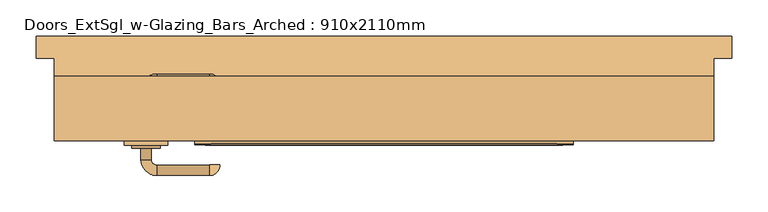
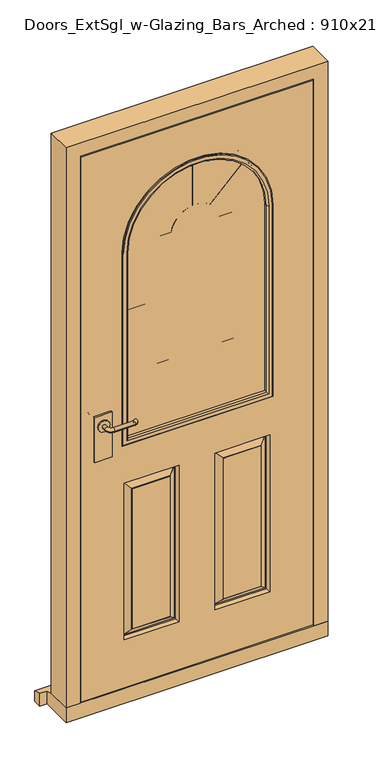
"""IFC4 building model written with IfcOpenShell, lengths in millimetres: door geometry, Doors_ExtSgl_w-Glazing_Bars_Arched : 910x2110mm."""

from ifc_helpers import new_model, si_unit, point, frame, frame_2d, origin, place, context, project, spatial, polyline, circle_curve, ellipse_curve, trimmed, segment, composite_curve, outline, extrude, faceted_brep, source, transform, mapped, element, save
from ifc_brep_helpers import plane_surface, cylinder_surface, revolved_surface, advanced_brep


def doors_extsgl_w_glazing_bars_arched_910x2110mm_1ab485ba(model_context):
    return source(origin(), model_context, "Body", "SolidModel", [
        extrude(outline(composite_curve([segment(trimmed(circle_curve(frame_2d((1050.0, -328.5)), 20.0), [point((1050.0, -348.5))], [point((1050.0, -308.5))], False, "CARTESIAN"), True, "CONTINUOUS"), segment(trimmed(circle_curve(frame_2d((1050.0, -328.5)), 20.0), [point((1050.0, -308.5))], [point((1050.0, -348.5))], False, "CARTESIAN"), True, "CONTINUOUS")], self_intersect=False)), frame((0.0, -22.9929895, 0.0), z_axis=(0.0, 1.0, 0.0), x_axis=(0.0, 0.0, 1.0)), (0.0, 0.0, 1.0), 4.5929895),
        advanced_brep(
        [(-321.5, -22.9929895, 1050.0), (-335.5, -22.9929895, 1050.0), (-335.5, -38.4, 1050.0), (-321.5, -38.4, 1050.0), (-313.5, -60.4, 1050.0), (-313.5, -46.4, 1050.0), (-241.5, -60.4, 1050.0), (-241.5, -46.4, 1050.0), (-240.5, -45.4, 1050.0), (-226.5, -45.4, 1050.0)],
        [
            (0, 1, circle_curve(frame((-328.5, -22.9929895, 1050.0), z_axis=(0.0, 1.0, 0.0), x_axis=(-1.0, 0.0, 0.0)), 7.0)),
            (1, 0, circle_curve(frame((-328.5, -22.9929895, 1050.0), z_axis=(0.0, 1.0, 0.0), x_axis=(-1.0, 0.0, 0.0)), 7.0)),
            (1, 2),
            (2, 3, circle_curve(frame((-328.5, -38.4, 1050.0), z_axis=(0.0, 1.0, 0.0), x_axis=(-1.0, 0.0, 0.0)), 7.0)),
            (3, 0),
            (3, 2, circle_curve(frame((-328.5, -38.4, 1050.0), z_axis=(0.0, 1.0, 0.0), x_axis=(-1.0, 0.0, 0.0)), 7.0)),
            (4, 5, circle_curve(frame((-313.5, -53.4, 1050.0), z_axis=(-1.0, 0.0, 0.0), x_axis=(0.0, -1.0, 0.0)), 7.0)),
            (5, 3, circle_curve(frame((-313.5, -38.4, 1050.0), z_axis=(0.0, 0.0, -1.0), x_axis=(-1.0, 0.0, 0.0)), 8.0)),
            (2, 4, circle_curve(frame((-313.5, -38.4, 1050.0), z_axis=(0.0, 0.0, 1.0), x_axis=(-1.0, 0.0, 0.0)), 22.0)),
            (5, 4, circle_curve(frame((-313.5, -53.4, 1050.0), z_axis=(-1.0, 0.0, 0.0), x_axis=(0.0, -1.0, 0.0)), 7.0)),
            (4, 6),
            (6, 7, circle_curve(frame((-241.5, -53.4, 1050.0), z_axis=(-1.0, 0.0, 0.0), x_axis=(0.0, -1.0, 0.0)), 7.0)),
            (7, 5),
            (7, 6, circle_curve(frame((-241.5, -53.4, 1050.0), z_axis=(-1.0, 0.0, 0.0), x_axis=(0.0, -1.0, 0.0)), 7.0)),
            (8, 9, circle_curve(frame((-233.5, -45.4, 1050.0), z_axis=(0.0, 1.0, 0.0), x_axis=(1.0, 0.0, 0.0)), 7.0)),
            (9, 8, circle_curve(frame((-233.5, -45.4, 1050.0), z_axis=(0.0, 1.0, 0.0), x_axis=(1.0, 0.0, 0.0)), 7.0)),
            (8, 7, circle_curve(frame((-241.5, -45.4, 1050.0), z_axis=(0.0, 0.0, -1.0), x_axis=(0.0, -1.0, 0.0)), 1.0)),
            (6, 9, circle_curve(frame((-241.5, -45.4, 1050.0), z_axis=(0.0, 0.0, 1.0), x_axis=(0.0, -1.0, 0.0)), 15.0)),
        ],
        [
            plane_surface(frame((-328.5, -22.9929895, 1050.0), z_axis=(0.0, 1.0, 0.0), x_axis=(0.0, 0.0, 1.0))),
            cylinder_surface(frame((-328.5, -22.9929895, 1050.0), z_axis=(0.0, 1.0, 0.0), x_axis=(-1.0, 0.0, 0.0)), 7.0),
            revolved_surface(trimmed(ellipse_curve(frame((-328.5, -38.4, 1050.0), z_axis=(0.0, -1.0, 0.0), x_axis=(-1.0, 0.0, 0.0)), 7.0, 7.0), [point((-321.5, -38.4, 1050.0))], [point((-335.5, -38.4, 1050.0))], True, "CARTESIAN"), (-313.5, -38.4, 1050.0), (0.0, 0.0, -1.0)),
            revolved_surface(trimmed(ellipse_curve(frame((-328.5, -38.4, 1050.0), z_axis=(0.0, -1.0, 0.0), x_axis=(-1.0, 0.0, 0.0)), 7.0, 7.0), [point((-335.5, -38.4, 1050.0))], [point((-321.5, -38.4, 1050.0))], True, "CARTESIAN"), (-313.5, -38.4, 1050.0), (0.0, 0.0, -1.0)),
            cylinder_surface(frame((-313.5, -53.4, 1050.0), z_axis=(-1.0, 0.0, 0.0), x_axis=(0.0, -1.0, 0.0)), 7.0),
            plane_surface(frame((-233.5, -45.4, 1050.0), z_axis=(0.0, 1.0, 0.0), x_axis=(0.0, 0.0, 1.0))),
            revolved_surface(trimmed(ellipse_curve(frame((-241.5, -53.4, 1050.0), z_axis=(1.0, 0.0, 0.0), x_axis=(0.0, -1.0, 0.0)), 7.0, 7.0), [point((-241.5, -46.4, 1050.0))], [point((-241.5, -60.4, 1050.0))], True, "CARTESIAN"), (-241.5, -45.4, 1050.0), (0.0, 0.0, -1.0)),
            revolved_surface(trimmed(ellipse_curve(frame((-241.5, -53.4, 1050.0), z_axis=(1.0, 0.0, 0.0), x_axis=(0.0, -1.0, 0.0)), 7.0, 7.0), [point((-241.5, -60.4, 1050.0))], [point((-241.5, -46.4, 1050.0))], True, "CARTESIAN"), (-241.5, -45.4, 1050.0), (0.0, 0.0, -1.0)),
        ],
        [
            (0, [[1, 2]]),
            (1, [[3, 4, 5, -2]]),
            (1, [[-5, 6, -3, -1]]),
            (2, [[7, 8, -4, 9]]),
            (3, [[10, -9, -6, -8]]),
            (4, [[11, 12, 13, -7]]),
            (4, [[-13, 14, -11, -10]]),
            (5, [[15, 16]]),
            (6, [[-15, 17, -12, 18]]),
            (7, [[-16, -18, -14, -17]]),
        ],
    ),
        extrude(outline(polyline([(-298.5, -12.4), (-298.5, -18.4), (-358.5, -18.4), (-358.5, -12.4), (-298.5, -12.4)])), frame((0.0, 0.0, 925.0), z_axis=(0.0, 0.0, 1.0), x_axis=(1.0, 0.0, 0.0)), (0.0, 0.0, 1.0), 165.0),
        extrude(outline(composite_curve([segment(trimmed(circle_curve(frame_2d((1050.0, -328.5)), 20.0), [point((1050.0, -348.5))], [point((1050.0, -308.5))], False, "CARTESIAN"), True, "CONTINUOUS"), segment(trimmed(circle_curve(frame_2d((1050.0, -328.5)), 20.0), [point((1050.0, -308.5))], [point((1050.0, -348.5))], False, "CARTESIAN"), True, "CONTINUOUS")], self_intersect=False)), frame((0.0, 37.6, 0.0), z_axis=(0.0, 1.0, 0.0), x_axis=(0.0, 0.0, 1.0)), (0.0, 0.0, 1.0), 4.5929895),
        advanced_brep(
        [(-321.5, 42.1929895, 1050.0), (-335.5, 42.1929895, 1050.0), (-321.5, 57.6, 1050.0), (-335.5, 57.6, 1050.0), (-313.5, 79.6, 1050.0), (-313.5, 65.6, 1050.0), (-241.5, 65.6, 1050.0), (-241.5, 79.6, 1050.0), (-240.5, 64.6, 1050.0), (-226.5, 64.6, 1050.0)],
        [
            (0, 1, circle_curve(frame((-328.5, 42.1929895, 1050.0), z_axis=(0.0, -1.0, 0.0), x_axis=(-1.0, 0.0, 0.0)), 7.0)),
            (1, 0, circle_curve(frame((-328.5, 42.1929895, 1050.0), z_axis=(0.0, -1.0, 0.0), x_axis=(-1.0, 0.0, 0.0)), 7.0)),
            (0, 2),
            (2, 3, circle_curve(frame((-328.5, 57.6, 1050.0), z_axis=(0.0, -1.0, 0.0), x_axis=(-1.0, 0.0, 0.0)), 7.0)),
            (3, 1),
            (3, 2, circle_curve(frame((-328.5, 57.6, 1050.0), z_axis=(0.0, -1.0, 0.0), x_axis=(-1.0, 0.0, 0.0)), 7.0)),
            (4, 3, circle_curve(frame((-313.5, 57.6, 1050.0), z_axis=(0.0, 0.0, 1.0), x_axis=(-1.0, 0.0, 0.0)), 22.0)),
            (2, 5, circle_curve(frame((-313.5, 57.6, 1050.0), z_axis=(0.0, 0.0, -1.0), x_axis=(-1.0, 0.0, 0.0)), 8.0)),
            (5, 4, circle_curve(frame((-313.5, 72.6, 1050.0), z_axis=(-1.0, 0.0, 0.0), x_axis=(0.0, 1.0, 0.0)), 7.0)),
            (4, 5, circle_curve(frame((-313.5, 72.6, 1050.0), z_axis=(-1.0, 0.0, 0.0), x_axis=(0.0, 1.0, 0.0)), 7.0)),
            (5, 6),
            (6, 7, circle_curve(frame((-241.5, 72.6, 1050.0), z_axis=(-1.0, 0.0, 0.0), x_axis=(0.0, 1.0, 0.0)), 7.0)),
            (7, 4),
            (7, 6, circle_curve(frame((-241.5, 72.6, 1050.0), z_axis=(-1.0, 0.0, 0.0), x_axis=(0.0, 1.0, 0.0)), 7.0)),
            (8, 9, circle_curve(frame((-233.5, 64.6, 1050.0), z_axis=(0.0, -1.0, 0.0), x_axis=(1.0, 0.0, 0.0)), 7.0)),
            (9, 8, circle_curve(frame((-233.5, 64.6, 1050.0), z_axis=(0.0, -1.0, 0.0), x_axis=(1.0, 0.0, 0.0)), 7.0)),
            (9, 7, circle_curve(frame((-241.5, 64.6, 1050.0), z_axis=(0.0, 0.0, 1.0), x_axis=(0.0, 1.0, 0.0)), 15.0)),
            (6, 8, circle_curve(frame((-241.5, 64.6, 1050.0), z_axis=(0.0, 0.0, -1.0), x_axis=(0.0, 1.0, 0.0)), 1.0)),
        ],
        [
            plane_surface(frame((-328.5, 42.1929895, 1050.0), z_axis=(0.0, -1.0, 0.0), x_axis=(0.0, 0.0, 1.0))),
            cylinder_surface(frame((-328.5, 42.1929895, 1050.0), z_axis=(0.0, -1.0, 0.0), x_axis=(-1.0, 0.0, 0.0)), 7.0),
            revolved_surface(trimmed(ellipse_curve(frame((-328.5, 57.6, 1050.0), z_axis=(0.0, -1.0, 0.0), x_axis=(-1.0, 0.0, 0.0)), 7.0, 7.0), [point((-321.5, 57.6, 1050.0))], [point((-335.5, 57.6, 1050.0))], True, "CARTESIAN"), (-313.5, 57.6, 1050.0), (0.0, 0.0, -1.0)),
            revolved_surface(trimmed(ellipse_curve(frame((-328.5, 57.6, 1050.0), z_axis=(0.0, -1.0, 0.0), x_axis=(-1.0, 0.0, 0.0)), 7.0, 7.0), [point((-335.5, 57.6, 1050.0))], [point((-321.5, 57.6, 1050.0))], True, "CARTESIAN"), (-313.5, 57.6, 1050.0), (0.0, 0.0, -1.0)),
            cylinder_surface(frame((-313.5, 72.6, 1050.0), z_axis=(-1.0, 0.0, 0.0), x_axis=(0.0, 1.0, 0.0)), 7.0),
            plane_surface(frame((-233.5, 64.6, 1050.0), z_axis=(0.0, -1.0, 0.0), x_axis=(0.0, 0.0, 1.0))),
            revolved_surface(trimmed(ellipse_curve(frame((-241.5, 72.6, 1050.0), z_axis=(-1.0, 0.0, 0.0), x_axis=(0.0, 1.0, 0.0)), 7.0, 7.0), [point((-241.5, 65.6, 1050.0))], [point((-241.5, 79.6, 1050.0))], True, "CARTESIAN"), (-241.5, 64.6, 1050.0), (0.0, 0.0, -1.0)),
            revolved_surface(trimmed(ellipse_curve(frame((-241.5, 72.6, 1050.0), z_axis=(-1.0, 0.0, 0.0), x_axis=(0.0, 1.0, 0.0)), 7.0, 7.0), [point((-241.5, 79.6, 1050.0))], [point((-241.5, 65.6, 1050.0))], True, "CARTESIAN"), (-241.5, 64.6, 1050.0), (0.0, 0.0, -1.0)),
        ],
        [
            (0, [[1, 2]]),
            (1, [[-1, 3, 4, 5]]),
            (1, [[-2, -5, 6, -3]]),
            (2, [[7, -4, 8, 9]]),
            (3, [[-8, -6, -7, 10]]),
            (4, [[-9, 11, 12, 13]]),
            (4, [[-10, -13, 14, -11]]),
            (5, [[15, 16]]),
            (6, [[17, -12, 18, -16]]),
            (7, [[-18, -14, -17, -15]]),
        ],
    ),
        extrude(outline(polyline([(-298.5, 31.6), (-358.5, 31.6), (-358.5, 37.6), (-298.5, 37.6), (-298.5, 31.6)])), frame((0.0, 0.0, 925.0), z_axis=(0.0, 0.0, 1.0), x_axis=(1.0, 0.0, 0.0)), (0.0, 0.0, 1.0), 165.0),
        faceted_brep([(384.5, 76.6, 54.5), (455.0, 76.6, 54.5), (455.0, -12.4, 54.5), (406.5, -12.4, 54.5), (406.5, 34.6, 54.5), (384.5, 34.6, 54.5), (384.5, 76.6, 2039.5), (-384.5, 76.6, 2039.5), (-384.5, 76.6, 54.5), (-455.0, 76.6, 54.5), (-455.0, 76.6, 2110.0), (455.0, 76.6, 2110.0), (455.0, -12.4, 2110.0), (-455.0, -12.4, 2110.0), (-455.0, -12.4, 54.5), (-406.5, -12.4, 54.5), (-406.5, -12.4, 2061.5), (406.5, -12.4, 2061.5), (406.5, 34.6, 2061.5), (-406.5, 34.6, 2061.5), (-406.5, 34.6, 54.5), (-384.5, 34.6, 54.5), (-384.5, 34.6, 2039.5), (384.5, 34.6, 2039.5)], [[[0, 1, 2, 3, 4, 5]], [[1, 0, 6, 7, 8, 9, 10, 11]], [[2, 1, 11, 12]], [[3, 2, 12, 13, 14, 15, 16, 17]], [[4, 3, 17, 18]], [[5, 4, 18, 19, 20, 21, 22, 23]], [[0, 5, 23, 6]], [[8, 7, 22, 21]], [[9, 8, 21, 20, 15, 14]], [[10, 9, 14, 13]], [[16, 15, 20, 19]], [[11, 10, 13, 12]], [[17, 16, 19, 18]], [[7, 6, 23, 22]]]),
        advanced_brep(
        [(403.5, -12.4, 58.5), (403.5, -12.4, 2058.5), (-404.4250294, -12.4, 2058.5), (-404.4250294, -12.4, 58.5), (-253.5, -12.4, 958.5), (-253.5, -12.4, 1655.0), (253.5, -12.4, 1655.0), (253.5, -12.4, 958.5), (-62.5, -12.4, 808.5), (-62.5, -12.4, 233.5), (-253.5, -12.4, 233.5), (-253.5, -12.4, 808.5), (253.5, -12.4, 808.5), (253.5, -12.4, 233.5), (62.5, -12.4, 233.5), (62.5, -12.4, 808.5), (-92.5, -12.4, 263.5), (-92.5, -12.4, 778.5), (-223.5, -12.4, 778.5), (-223.5, -12.4, 263.5), (223.5, -12.4, 263.5), (223.5, -12.4, 778.5), (92.5, -12.4, 778.5), (92.5, -12.4, 263.5), (403.5, 31.6, 58.5), (-404.4250294, 31.6, 58.5), (-404.4250294, 31.6, 2058.5), (403.5, 31.6, 2058.5), (-253.5, 31.6, 958.5), (253.5, 31.6, 958.5), (253.5, 31.6, 1655.0), (-253.5, 31.6, 1655.0), (62.5, 31.6, 808.5), (62.5, 31.6, 233.5), (253.5, 31.6, 233.5), (253.5, 31.6, 808.5), (-253.5, 31.6, 808.5), (-253.5, 31.6, 233.5), (-62.5, 31.6, 233.5), (-62.5, 31.6, 808.5), (92.5, 31.6, 263.5), (92.5, 31.6, 778.5), (223.5, 31.6, 778.5), (223.5, 31.6, 263.5), (-223.5, 31.6, 263.5), (-223.5, 31.6, 778.5), (-92.5, 31.6, 778.5), (-92.5, 31.6, 263.5), (65.5, 16.6, 805.5), (65.5, 16.6, 236.5), (90.5, 30.6, 780.5), (90.5, 30.6, 261.5), (70.5, 16.6, 241.5), (70.5, 16.6, 800.5), (92.5, 30.6, 263.5), (92.5, 30.6, 778.5), (250.5, 16.6, 236.5), (225.5, 30.6, 261.5), (245.5, 16.6, 241.5), (223.5, 30.6, 263.5), (250.5, 16.6, 805.5), (225.5, 30.6, 780.5), (245.5, 16.6, 800.5), (223.5, 30.6, 778.5), (-250.5, 16.6, 805.5), (-250.5, 16.6, 236.5), (-225.5, 30.6, 780.5), (-225.5, 30.6, 261.5), (-245.5, 16.6, 241.5), (-245.5, 16.6, 800.5), (-223.5, 30.6, 263.5), (-223.5, 30.6, 778.5), (-65.5, 16.6, 236.5), (-90.5, 30.6, 261.5), (-70.5, 16.6, 241.5), (-92.5, 30.6, 263.5), (-65.5, 16.6, 805.5), (-90.5, 30.6, 780.5), (-70.5, 16.6, 800.5), (-92.5, 30.6, 778.5), (-92.5, -11.4, 263.5), (-92.5, -11.4, 778.5), (-70.5, 2.6, 241.5), (-70.5, 2.6, 800.5), (-90.5, -11.4, 780.5), (-90.5, -11.4, 261.5), (-65.5, 2.6, 805.5), (-65.5, 2.6, 236.5), (-223.5, -11.4, 778.5), (-245.5, 2.6, 800.5), (-225.5, -11.4, 780.5), (-250.5, 2.6, 805.5), (-223.5, -11.4, 263.5), (-245.5, 2.6, 241.5), (-225.5, -11.4, 261.5), (-250.5, 2.6, 236.5), (250.5, 2.6, 805.5), (250.5, 2.6, 236.5), (225.5, -11.4, 780.5), (225.5, -11.4, 261.5), (245.5, 2.6, 241.5), (245.5, 2.6, 800.5), (223.5, -11.4, 263.5), (223.5, -11.4, 778.5), (65.5, 2.6, 236.5), (90.5, -11.4, 261.5), (70.5, 2.6, 241.5), (92.5, -11.4, 263.5), (65.5, 2.6, 805.5), (90.5, -11.4, 780.5), (70.5, 2.6, 800.5), (92.5, -11.4, 778.5)],
        [
            (0, 1),
            (1, 2),
            (2, 3),
            (3, 0),
            (4, 5),
            (5, 6, circle_curve(frame((0.0, -12.4, 1655.0), z_axis=(0.0, 1.0, 0.0), x_axis=(1.0, 0.0, 0.0)), 253.5)),
            (6, 7),
            (7, 4),
            (8, 9),
            (9, 10),
            (10, 11),
            (11, 8),
            (12, 13),
            (13, 14),
            (14, 15),
            (15, 12),
            (16, 17),
            (17, 18),
            (18, 19),
            (19, 16),
            (20, 21),
            (21, 22),
            (22, 23),
            (23, 20),
            (24, 25),
            (25, 26),
            (26, 27),
            (27, 24),
            (28, 29),
            (29, 30),
            (30, 31, circle_curve(frame((0.0, 31.6, 1655.0), z_axis=(0.0, -1.0, 0.0), x_axis=(1.0, 0.0, 0.0)), 253.5)),
            (31, 28),
            (32, 33),
            (33, 34),
            (34, 35),
            (35, 32),
            (36, 37),
            (37, 38),
            (38, 39),
            (39, 36),
            (40, 41),
            (41, 42),
            (42, 43),
            (43, 40),
            (44, 45),
            (45, 46),
            (46, 47),
            (47, 44),
            (0, 24),
            (27, 1),
            (26, 2),
            (25, 3),
            (4, 28),
            (31, 5),
            (30, 6),
            (29, 7),
            (48, 49),
            (49, 33),
            (32, 48),
            (50, 51),
            (51, 52),
            (52, 53),
            (53, 50),
            (40, 54),
            (54, 55),
            (55, 41),
            (49, 56),
            (56, 34),
            (51, 57),
            (57, 58),
            (58, 52),
            (43, 59),
            (59, 54),
            (56, 60),
            (60, 35),
            (57, 61),
            (61, 62),
            (62, 58),
            (42, 63),
            (63, 59),
            (60, 48),
            (62, 53),
            (61, 50),
            (63, 55),
            (64, 65),
            (65, 37),
            (36, 64),
            (66, 67),
            (67, 68),
            (68, 69),
            (69, 66),
            (44, 70),
            (70, 71),
            (71, 45),
            (65, 72),
            (72, 38),
            (67, 73),
            (73, 74),
            (74, 68),
            (47, 75),
            (75, 70),
            (72, 76),
            (76, 39),
            (73, 77),
            (77, 78),
            (78, 74),
            (46, 79),
            (79, 75),
            (76, 64),
            (78, 69),
            (77, 66),
            (79, 71),
            (80, 81),
            (81, 17),
            (16, 80),
            (82, 83),
            (83, 84),
            (84, 85),
            (85, 82),
            (8, 86),
            (86, 87),
            (87, 9),
            (81, 88),
            (88, 18),
            (83, 89),
            (89, 90),
            (90, 84),
            (11, 91),
            (91, 86),
            (88, 92),
            (92, 19),
            (89, 93),
            (93, 94),
            (94, 90),
            (10, 95),
            (95, 91),
            (92, 80),
            (94, 85),
            (93, 82),
            (95, 87),
            (96, 97),
            (97, 13),
            (12, 96),
            (98, 99),
            (99, 100),
            (100, 101),
            (101, 98),
            (20, 102),
            (102, 103),
            (103, 21),
            (97, 104),
            (104, 14),
            (99, 105),
            (105, 106),
            (106, 100),
            (23, 107),
            (107, 102),
            (104, 108),
            (108, 15),
            (105, 109),
            (109, 110),
            (110, 106),
            (22, 111),
            (111, 107),
            (108, 96),
            (110, 101),
            (109, 98),
            (111, 103),
        ],
        [
            plane_surface(frame((403.5, -12.4, 58.5), z_axis=(0.0, -1.0, 0.0), x_axis=(0.0, 0.0, 1.0))),
            plane_surface(frame((403.5, 31.6, 58.5), z_axis=(0.0, 1.0, 0.0), x_axis=(0.0, 0.0, -1.0))),
            plane_surface(frame((403.5, -12.4, 58.5), z_axis=(1.0, 0.0, 0.0), x_axis=(0.0, 1.0, 0.0))),
            plane_surface(frame((403.5, -12.4, 2058.5), z_axis=(0.0, 0.0, 1.0), x_axis=(0.0, 1.0, 0.0))),
            plane_surface(frame((-404.4250294, -12.4, 2058.5), z_axis=(-1.0, 0.0, 0.0), x_axis=(0.0, 1.0, 0.0))),
            plane_surface(frame((-404.4250294, -12.4, 58.5), z_axis=(0.0, 0.0, -1.0), x_axis=(0.0, 1.0, 0.0))),
            plane_surface(frame((-253.5, -12.4, 958.5), z_axis=(1.0, 0.0, 0.0), x_axis=(0.0, 1.0, 0.0))),
            revolved_surface(polyline([(253.5, 31.6, 1655.0), (253.5, -12.4, 1655.0)]), (0.0, -12.4, 1655.0), (0.0, 1.0, 0.0)),
            plane_surface(frame((253.5, -12.4, 1655.0), z_axis=(-1.0, 0.0, 0.0), x_axis=(0.0, 1.0, 0.0))),
            plane_surface(frame((253.5, -12.4, 958.5), z_axis=(0.0, 0.0, 1.0), x_axis=(0.0, 1.0, 0.0))),
            plane_surface(frame((62.5, 31.6, 808.5), z_axis=(0.9805806756909202, 0.19611613513818407, 0.0), x_axis=(0.0, 0.0, -1.0))),
            plane_surface(frame((70.5, 16.6, 800.5), z_axis=(-0.5734623443633278, 0.8192319205190408, 0.0), x_axis=(0.0, 0.0, -1.0))),
            plane_surface(frame((92.5, 30.6, 778.5), z_axis=(-1.0, 0.0, 0.0), x_axis=(0.0, 0.0, -1.0))),
            plane_surface(frame((62.5, 31.6, 233.5), z_axis=(0.0, 0.19611613513818724, 0.9805806756909196), x_axis=(1.0, 0.0, 0.0))),
            plane_surface(frame((70.5, 16.6, 241.5), z_axis=(0.0, 0.819231920519039, -0.5734623443633305), x_axis=(1.0, 0.0, 0.0))),
            plane_surface(frame((92.5, 30.6, 263.5), z_axis=(0.0, 0.0, -1.0), x_axis=(1.0, 0.0, 0.0))),
            plane_surface(frame((253.5, 31.6, 233.5), z_axis=(-0.9805806756909189, 0.19611613513819037, 0.0), x_axis=(0.0, 0.0, 1.0))),
            plane_surface(frame((245.5, 16.6, 241.5), z_axis=(0.5734623443633332, 0.819231920519037, 0.0), x_axis=(0.0, 0.0, 1.0))),
            plane_surface(frame((223.5, 30.6, 263.5), z_axis=(1.0, 0.0, 0.0), x_axis=(0.0, 0.0, 1.0))),
            plane_surface(frame((253.5, 31.6, 808.5), z_axis=(0.0, 0.1961161351381872, -0.9805806756909196), x_axis=(-1.0, 0.0, 0.0))),
            plane_surface(frame((250.5, 16.6, 805.5), z_axis=(0.0, 1.0, 0.0), x_axis=(-1.0, 0.0, 0.0))),
            plane_surface(frame((245.5, 16.6, 800.5), z_axis=(0.0, 0.8192319205190389, 0.5734623443633305), x_axis=(-1.0, 0.0, 0.0))),
            plane_surface(frame((225.5, 30.6, 780.5), z_axis=(0.0, 1.0, 0.0), x_axis=(-1.0, 0.0, 0.0))),
            plane_surface(frame((223.5, 30.6, 778.5), z_axis=(0.0, 0.0, 1.0), x_axis=(-1.0, 0.0, 0.0))),
            plane_surface(frame((-253.5, 31.6, 808.5), z_axis=(0.9805806756909202, 0.19611613513818407, 0.0), x_axis=(0.0, 0.0, -1.0))),
            plane_surface(frame((-245.5, 16.6, 800.5), z_axis=(-0.5734623443633278, 0.8192319205190408, 0.0), x_axis=(0.0, 0.0, -1.0))),
            plane_surface(frame((-223.5, 30.6, 778.5), z_axis=(-1.0, 0.0, 0.0), x_axis=(0.0, 0.0, -1.0))),
            plane_surface(frame((-253.5, 31.6, 233.5), z_axis=(0.0, 0.19611613513818724, 0.9805806756909196), x_axis=(1.0, 0.0, 0.0))),
            plane_surface(frame((-245.5, 16.6, 241.5), z_axis=(0.0, 0.819231920519039, -0.5734623443633305), x_axis=(1.0, 0.0, 0.0))),
            plane_surface(frame((-223.5, 30.6, 263.5), z_axis=(0.0, 0.0, -1.0), x_axis=(1.0, 0.0, 0.0))),
            plane_surface(frame((-62.5, 31.6, 233.5), z_axis=(-0.9805806756909189, 0.1961161351381904, 0.0), x_axis=(0.0, 0.0, 1.0))),
            plane_surface(frame((-70.5, 16.6, 241.5), z_axis=(0.5734623443633332, 0.8192319205190371, 0.0), x_axis=(0.0, 0.0, 1.0))),
            plane_surface(frame((-92.5, 30.6, 263.5), z_axis=(1.0, 0.0, 0.0), x_axis=(0.0, 0.0, 1.0))),
            plane_surface(frame((-62.5, 31.6, 808.5), z_axis=(0.0, 0.19611613513818724, -0.9805806756909196), x_axis=(-1.0, 0.0, 0.0))),
            plane_surface(frame((-65.5, 16.6, 805.5), z_axis=(0.0, 1.0, 0.0), x_axis=(-1.0, 0.0, 0.0))),
            plane_surface(frame((-70.5, 16.6, 800.5), z_axis=(0.0, 0.819231920519039, 0.5734623443633305), x_axis=(-1.0, 0.0, 0.0))),
            plane_surface(frame((-90.5, 30.6, 780.5), z_axis=(0.0, 1.0, 0.0), x_axis=(-1.0, 0.0, 0.0))),
            plane_surface(frame((-92.5, 30.6, 778.5), z_axis=(0.0, 0.0, 1.0), x_axis=(-1.0, 0.0, 0.0))),
            plane_surface(frame((-92.5, -12.4, 263.5), z_axis=(1.0, 0.0, 0.0), x_axis=(0.0, 0.0, 1.0))),
            plane_surface(frame((-90.5, -11.4, 261.5), z_axis=(0.5734623443633226, -0.8192319205190446, 0.0), x_axis=(0.0, 0.0, 1.0))),
            plane_surface(frame((-65.5, 2.6, 236.5), z_axis=(-0.9805806756909214, -0.19611613513817774, 0.0), x_axis=(0.0, 0.0, 1.0))),
            plane_surface(frame((-92.5, -12.4, 778.5), z_axis=(0.0, 0.0, 1.0), x_axis=(-1.0, 0.0, 0.0))),
            plane_surface(frame((-90.5, -11.4, 780.5), z_axis=(0.0, -0.8192319205190427, 0.5734623443633252), x_axis=(-1.0, 0.0, 0.0))),
            plane_surface(frame((-65.5, 2.6, 805.5), z_axis=(0.0, -0.1961161351381809, -0.9805806756909208), x_axis=(-1.0, 0.0, 0.0))),
            plane_surface(frame((-223.5, -12.4, 778.5), z_axis=(-1.0, 0.0, 0.0), x_axis=(0.0, 0.0, -1.0))),
            plane_surface(frame((-225.5, -11.4, 780.5), z_axis=(-0.5734623443633279, -0.8192319205190408, 0.0), x_axis=(0.0, 0.0, -1.0))),
            plane_surface(frame((-250.5, 2.6, 805.5), z_axis=(0.9805806756909202, -0.1961161351381841, 0.0), x_axis=(0.0, 0.0, -1.0))),
            plane_surface(frame((-223.5, -12.4, 263.5), z_axis=(0.0, 0.0, -1.0), x_axis=(1.0, 0.0, 0.0))),
            plane_surface(frame((-223.5, -11.4, 263.5), z_axis=(0.0, -1.0, 0.0), x_axis=(1.0, 0.0, 0.0))),
            plane_surface(frame((-225.5, -11.4, 261.5), z_axis=(0.0, -0.8192319205190427, -0.5734623443633252), x_axis=(1.0, 0.0, 0.0))),
            plane_surface(frame((-245.5, 2.6, 241.5), z_axis=(0.0, -1.0, 0.0), x_axis=(1.0, 0.0, 0.0))),
            plane_surface(frame((-250.5, 2.6, 236.5), z_axis=(0.0, -0.19611613513818094, 0.9805806756909209), x_axis=(1.0, 0.0, 0.0))),
            plane_surface(frame((253.5, -12.4, 808.5), z_axis=(-0.9805806756909202, -0.19611613513818407, 0.0), x_axis=(0.0, 0.0, -1.0))),
            plane_surface(frame((245.5, 2.6, 800.5), z_axis=(0.5734623443633278, -0.8192319205190408, 0.0), x_axis=(0.0, 0.0, -1.0))),
            plane_surface(frame((223.5, -11.4, 778.5), z_axis=(1.0, 0.0, 0.0), x_axis=(0.0, 0.0, -1.0))),
            plane_surface(frame((253.5, -12.4, 233.5), z_axis=(0.0, -0.19611613513818724, 0.9805806756909196), x_axis=(-1.0, 0.0, 0.0))),
            plane_surface(frame((245.5, 2.6, 241.5), z_axis=(0.0, -0.819231920519039, -0.5734623443633305), x_axis=(-1.0, 0.0, 0.0))),
            plane_surface(frame((223.5, -11.4, 263.5), z_axis=(0.0, 0.0, -1.0), x_axis=(-1.0, 0.0, 0.0))),
            plane_surface(frame((62.5, -12.4, 233.5), z_axis=(0.9805806756909189, -0.19611613513819046, 0.0), x_axis=(0.0, 0.0, 1.0))),
            plane_surface(frame((70.5, 2.6, 241.5), z_axis=(-0.5734623443633331, -0.8192319205190371, 0.0), x_axis=(0.0, 0.0, 1.0))),
            plane_surface(frame((92.5, -11.4, 263.5), z_axis=(-1.0, 0.0, 0.0), x_axis=(0.0, 0.0, 1.0))),
            plane_surface(frame((62.5, -12.4, 808.5), z_axis=(0.0, -0.1961161351381873, -0.9805806756909196), x_axis=(1.0, 0.0, 0.0))),
            plane_surface(frame((65.5, 2.6, 805.5), z_axis=(0.0, -1.0, 0.0), x_axis=(1.0, 0.0, 0.0))),
            plane_surface(frame((70.5, 2.6, 800.5), z_axis=(0.0, -0.819231920519039, 0.5734623443633304), x_axis=(1.0, 0.0, 0.0))),
            plane_surface(frame((90.5, -11.4, 780.5), z_axis=(0.0, -1.0, 0.0), x_axis=(1.0, 0.0, 0.0))),
            plane_surface(frame((92.5, -11.4, 778.5), z_axis=(0.0, 0.0, 1.0), x_axis=(1.0, 0.0, 0.0))),
        ],
        [
            (0, [[1, 2, 3, 4], [5, 6, 7, 8], [9, 10, 11, 12], [13, 14, 15, 16]]),
            (0, [[17, 18, 19, 20]]),
            (0, [[21, 22, 23, 24]]),
            (1, [[25, 26, 27, 28], [29, 30, 31, 32], [33, 34, 35, 36], [37, 38, 39, 40]]),
            (1, [[41, 42, 43, 44]]),
            (1, [[45, 46, 47, 48]]),
            (2, [[-1, 49, -28, 50]]),
            (3, [[-2, -50, -27, 51]]),
            (4, [[-3, -51, -26, 52]]),
            (5, [[-4, -52, -25, -49]]),
            (6, [[-5, 53, -32, 54]]),
            (7, [[-6, -54, -31, 55]]),
            (8, [[-7, -55, -30, 56]]),
            (9, [[-8, -56, -29, -53]]),
            (10, [[57, 58, -33, 59]]),
            (11, [[60, 61, 62, 63]]),
            (12, [[64, 65, 66, -41]]),
            (13, [[-58, 67, 68, -34]]),
            (14, [[-61, 69, 70, 71]]),
            (15, [[-64, -44, 72, 73]]),
            (16, [[-68, 74, 75, -35]]),
            (17, [[-70, 76, 77, 78]]),
            (18, [[-72, -43, 79, 80]]),
            (19, [[-59, -36, -75, 81]]),
            (20, [[-57, -81, -74, -67], [-62, -71, -78, 82]]),
            (21, [[-63, -82, -77, 83]]),
            (22, [[-60, -83, -76, -69], [-65, -73, -80, 84]]),
            (23, [[-66, -84, -79, -42]]),
            (24, [[85, 86, -37, 87]]),
            (25, [[88, 89, 90, 91]]),
            (26, [[92, 93, 94, -45]]),
            (27, [[-86, 95, 96, -38]]),
            (28, [[-89, 97, 98, 99]]),
            (29, [[-92, -48, 100, 101]]),
            (30, [[-96, 102, 103, -39]]),
            (31, [[-98, 104, 105, 106]]),
            (32, [[-100, -47, 107, 108]]),
            (33, [[-87, -40, -103, 109]]),
            (34, [[-85, -109, -102, -95], [-90, -99, -106, 110]]),
            (35, [[-91, -110, -105, 111]]),
            (36, [[-88, -111, -104, -97], [-93, -101, -108, 112]]),
            (37, [[-94, -112, -107, -46]]),
            (38, [[113, 114, -17, 115]]),
            (39, [[116, 117, 118, 119]]),
            (40, [[120, 121, 122, -9]]),
            (41, [[-114, 123, 124, -18]]),
            (42, [[-117, 125, 126, 127]]),
            (43, [[-120, -12, 128, 129]]),
            (44, [[-124, 130, 131, -19]]),
            (45, [[-126, 132, 133, 134]]),
            (46, [[-128, -11, 135, 136]]),
            (47, [[-115, -20, -131, 137]]),
            (48, [[-118, -127, -134, 138], [-113, -137, -130, -123]]),
            (49, [[-119, -138, -133, 139]]),
            (50, [[-121, -129, -136, 140], [-116, -139, -132, -125]]),
            (51, [[-122, -140, -135, -10]]),
            (52, [[141, 142, -13, 143]]),
            (53, [[144, 145, 146, 147]]),
            (54, [[148, 149, 150, -21]]),
            (55, [[-142, 151, 152, -14]]),
            (56, [[-145, 153, 154, 155]]),
            (57, [[-148, -24, 156, 157]]),
            (58, [[-152, 158, 159, -15]]),
            (59, [[-154, 160, 161, 162]]),
            (60, [[-156, -23, 163, 164]]),
            (61, [[-143, -16, -159, 165]]),
            (62, [[-141, -165, -158, -151], [-146, -155, -162, 166]]),
            (63, [[-147, -166, -161, 167]]),
            (64, [[-144, -167, -160, -153], [-149, -157, -164, 168]]),
            (65, [[-150, -168, -163, -22]]),
        ],
    ),
        faceted_brep([(480.0, 131.6, 0.0), (480.0, 131.6, 38.5947221), (480.0, 101.6, 47.2703282), (480.0, 101.6, 0.0), (-480.0, 131.6, 38.5947221), (-480.0, 131.6, 0.0), (-480.0, 101.6, 0.0), (-480.0, 101.6, 47.2703282), (455.0, 101.6, 0.0), (455.0, -12.4, 0.0), (-455.0, -12.4, 0.0), (-455.0, 101.6, 0.0), (-455.0, 101.6, 47.2703282), (-455.0, 76.6, 54.5), (455.0, 76.6, 54.5), (455.0, 101.6, 47.2703282), (-455.0, -12.4, 54.5), (455.0, -12.4, 54.5)], [[[0, 1, 2, 3]], [[4, 5, 6, 7]], [[5, 0, 3, 8, 9, 10, 11, 6]], [[1, 0, 5, 4]], [[1, 4, 7, 12, 13, 14, 15, 2]], [[13, 16, 17, 14]], [[16, 10, 9, 17]], [[12, 11, 10, 16, 13]], [[11, 12, 7, 6]], [[8, 15, 14, 17, 9]], [[15, 8, 3, 2]]]),
        extrude(outline(composite_curve([segment(polyline([(958.5, -253.5), (958.5, 253.5), (1655.0, 253.5)]), True, "CONTINUOUS"), segment(trimmed(circle_curve(frame_2d((1655.0, 0.0)), 253.5), [point((1655.0, 253.5))], [point((1655.0, -253.5))], False, "CARTESIAN"), True, "CONTINUOUS"), segment(polyline([(1655.0, -253.5), (958.5, -253.5)]), True, "CONTINUOUS")], self_intersect=False)), frame((0.0, -2.4, 0.0), z_axis=(0.0, 1.0, 0.0), x_axis=(0.0, 0.0, 1.0)), (0.0, 0.0, 1.0), 24.0),
        advanced_brep(
        [(-261.5, 35.6, 950.5), (-261.5, 31.6, 950.5), (-261.5, 31.6, 1655.0), (-261.5, 35.6, 1655.0), (-259.5, 37.6, 952.5), (-259.5, 37.6, 1655.0), (-241.5, 32.6, 970.5), (-246.5, 37.6, 965.5), (-246.5, 37.6, 1655.0), (-241.5, 32.6, 1655.0), (-241.5, 21.6, 970.5), (-241.5, 21.6, 1655.0), (-253.5, 31.6, 958.5), (-253.5, 21.6, 958.5), (-253.5, 21.6, 1655.0), (-253.5, 31.6, 1655.0), (261.5, 35.6, 1655.0), (261.5, 31.6, 1655.0), (259.5, 37.6, 1655.0), (259.5, 37.6, 952.5), (246.5, 37.6, 1655.0), (246.5, 37.6, 965.5), (241.5, 32.6, 1655.0), (241.5, 21.6, 1655.0), (253.5, 21.6, 1655.0), (253.5, 21.6, 958.5), (241.5, 21.6, 970.5), (253.5, 31.6, 1655.0), (261.5, 31.6, 950.5), (253.5, 31.6, 958.5), (261.5, 35.6, 950.5), (241.5, 32.6, 970.5)],
        [
            (0, 1),
            (1, 2),
            (2, 3),
            (3, 0),
            (4, 0, ellipse_curve(frame((-259.5, 35.6, 952.5), z_axis=(-0.7071067811865475, 0.0, 0.7071067811865475), x_axis=(-0.7071067811865472, 0.0, -0.7071067811865477)), 2.8284271, 2.0)),
            (3, 5, circle_curve(frame((-259.5, 35.6, 1655.0), z_axis=(0.0, 0.0, -1.0), x_axis=(-1.0, 0.0, 0.0)), 2.0)),
            (5, 4),
            (6, 7, ellipse_curve(frame((-246.5, 32.6, 965.5), z_axis=(-0.7071067811865475, 0.0, 0.7071067811865475), x_axis=(-0.7071067811865472, 0.0, -0.7071067811865477)), 7.0710678, 5.0)),
            (7, 8),
            (8, 9, circle_curve(frame((-246.5, 32.6, 1655.0), z_axis=(0.0, 0.0, -1.0), x_axis=(-1.0, 0.0, 0.0)), 5.0)),
            (9, 6),
            (10, 6),
            (9, 11),
            (11, 10),
            (12, 13),
            (13, 14),
            (14, 15),
            (15, 12),
            (16, 3, circle_curve(frame((0.0, 35.6, 1655.0), z_axis=(0.0, -1.0, 0.0), x_axis=(-1.0, 0.0, 0.0)), 261.5)),
            (2, 17, circle_curve(frame((0.0, 31.6, 1655.0), z_axis=(0.0, 1.0, 0.0), x_axis=(-1.0, 0.0, 0.0)), 261.5)),
            (17, 16),
            (18, 5, circle_curve(frame((0.0, 37.6, 1655.0), z_axis=(0.0, -1.0, 0.0), x_axis=(-1.0, 0.0, 0.0)), 259.5)),
            (16, 18, circle_curve(frame((259.5, 35.6, 1655.0), z_axis=(0.0, 0.0, 1.0), x_axis=(1.0, 0.0, 0.0)), 2.0)),
            (18, 19),
            (19, 4),
            (20, 8, circle_curve(frame((0.0, 37.6, 1655.0), z_axis=(0.0, -1.0, 0.0), x_axis=(-1.0, 0.0, 0.0)), 246.5)),
            (7, 21),
            (21, 20),
            (22, 9, circle_curve(frame((0.0, 32.6, 1655.0), z_axis=(0.0, -1.0, 0.0), x_axis=(-1.0, 0.0, 0.0)), 241.5)),
            (20, 22, circle_curve(frame((246.5, 32.6, 1655.0), z_axis=(0.0, 0.0, 1.0), x_axis=(1.0, 0.0, 0.0)), 5.0)),
            (23, 11, circle_curve(frame((0.0, 21.6, 1655.0), z_axis=(0.0, -1.0, 0.0), x_axis=(-1.0, 0.0, 0.0)), 241.5)),
            (22, 23),
            (24, 14, circle_curve(frame((0.0, 21.6, 1655.0), z_axis=(0.0, -1.0, 0.0), x_axis=(-1.0, 0.0, 0.0)), 253.5)),
            (13, 25),
            (25, 24),
            (23, 26),
            (26, 10),
            (27, 15, circle_curve(frame((0.0, 31.6, 1655.0), z_axis=(0.0, -1.0, 0.0), x_axis=(-1.0, 0.0, 0.0)), 253.5)),
            (24, 27),
            (1, 28),
            (28, 17),
            (27, 29),
            (29, 12),
            (28, 30),
            (30, 16),
            (30, 19, ellipse_curve(frame((259.5, 35.6, 952.5), z_axis=(0.7071067811865475, 0.0, 0.7071067811865475), x_axis=(-0.7071067811865475, 0.0, 0.7071067811865476)), 2.8284271, 2.0)),
            (21, 31, ellipse_curve(frame((246.5, 32.6, 965.5), z_axis=(0.7071067811865475, 0.0, 0.7071067811865475), x_axis=(-0.7071067811865475, 0.0, 0.7071067811865476)), 7.0710678, 5.0)),
            (31, 22),
            (31, 26),
            (25, 29),
            (0, 30),
            (6, 31),
        ],
        [
            plane_surface(frame((-261.5, 31.6, 950.5), z_axis=(-1.0, 0.0, 0.0), x_axis=(0.0, 0.0, 1.0))),
            cylinder_surface(frame((-259.5, 35.6, 958.5), z_axis=(0.0, 0.0, -1.0), x_axis=(-1.0, 0.0, 0.0)), 2.0),
            cylinder_surface(frame((-246.5, 32.6, 958.5), z_axis=(0.0, 0.0, -1.0), x_axis=(-1.0, 0.0, 0.0)), 5.0),
            plane_surface(frame((-241.5, 32.6, 970.5), z_axis=(1.0, 0.0, 0.0), x_axis=(0.0, 0.0, 1.0))),
            plane_surface(frame((-253.5, 21.6, 958.5), z_axis=(-1.0, 0.0, 0.0), x_axis=(0.0, 0.0, 1.0))),
            cylinder_surface(frame((0.0, 31.6, 1655.0), z_axis=(0.0, 1.0, 0.0), x_axis=(-1.0, 0.0, 0.0)), 261.5),
            revolved_surface(trimmed(ellipse_curve(frame((-259.5, 35.6, 1655.0), z_axis=(0.0, 0.0, -1.0), x_axis=(-1.0, 0.0, 0.0)), 2.0, 2.0), [point((-261.5, 35.6, 1655.0))], [point((-259.5, 37.6, 1655.0))], True, "CARTESIAN"), (0.0, 31.6, 1655.0), (0.0, 1.0, 0.0)),
            plane_surface(frame((0.0, 37.6, 1655.0), z_axis=(0.0, 1.0, 0.0), x_axis=(-1.0, 0.0, 0.0))),
            revolved_surface(trimmed(ellipse_curve(frame((-246.5, 32.6, 1655.0), z_axis=(0.0, 0.0, -1.0), x_axis=(-1.0, 0.0, 0.0)), 5.0, 5.0), [point((-246.5, 37.6, 1655.0))], [point((-241.5, 32.6, 1655.0))], True, "CARTESIAN"), (0.0, 31.6, 1655.0), (0.0, 1.0, 0.0)),
            revolved_surface(polyline([(-241.5, 32.6, 1655.0), (-241.5, 21.6, 1655.0)]), (0.0, 31.6, 1655.0), (0.0, 1.0, 0.0)),
            plane_surface(frame((0.0, 21.6, 1655.0), z_axis=(0.0, -1.0, 0.0), x_axis=(-1.0, 0.0, 0.0))),
            cylinder_surface(frame((0.0, 31.6, 1655.0), z_axis=(0.0, 1.0, 0.0), x_axis=(-1.0, 0.0, 0.0)), 253.5),
            plane_surface(frame((0.0, 31.6, 1655.0), z_axis=(0.0, -1.0, 0.0), x_axis=(-1.0, 0.0, 0.0))),
            plane_surface(frame((261.5, 31.6, 1655.0), z_axis=(1.0, 0.0, 0.0), x_axis=(0.0, 0.0, -1.0))),
            cylinder_surface(frame((259.5, 35.6, 1655.0), z_axis=(0.0, 0.0, 1.0), x_axis=(1.0, 0.0, 0.0)), 2.0),
            cylinder_surface(frame((246.5, 32.6, 1655.0), z_axis=(0.0, 0.0, 1.0), x_axis=(1.0, 0.0, 0.0)), 5.0),
            plane_surface(frame((241.5, 32.6, 1655.0), z_axis=(-1.0, 0.0, 0.0), x_axis=(0.0, 0.0, -1.0))),
            plane_surface(frame((253.5, 21.6, 1655.0), z_axis=(1.0, 0.0, 0.0), x_axis=(0.0, 0.0, -1.0))),
            plane_surface(frame((261.5, 31.6, 950.5), z_axis=(0.0, 0.0, -1.0), x_axis=(-1.0, 0.0, 0.0))),
            cylinder_surface(frame((253.5, 35.6, 952.5), z_axis=(1.0, 0.0, 0.0), x_axis=(0.0, 0.0, -1.0)), 2.0),
            cylinder_surface(frame((253.5, 32.6, 965.5), z_axis=(1.0, 0.0, 0.0), x_axis=(0.0, 0.0, -1.0)), 5.0),
            plane_surface(frame((241.5, 32.6, 970.5), z_axis=(0.0, 0.0, 1.0), x_axis=(-1.0, 0.0, 0.0))),
            plane_surface(frame((253.5, 21.6, 958.5), z_axis=(0.0, 0.0, -1.0), x_axis=(-1.0, 0.0, 0.0))),
        ],
        [
            (0, [[1, 2, 3, 4]]),
            (1, [[5, -4, 6, 7]]),
            (2, [[8, 9, 10, 11]]),
            (3, [[12, -11, 13, 14]]),
            (4, [[15, 16, 17, 18]]),
            (5, [[19, -3, 20, 21]]),
            (6, [[22, -6, -19, 23]]),
            (7, [[24, 25, -7, -22], [26, -9, 27, 28]]),
            (8, [[29, -10, -26, 30]]),
            (9, [[31, -13, -29, 32]]),
            (10, [[33, -16, 34, 35], [36, 37, -14, -31]]),
            (11, [[38, -17, -33, 39]]),
            (12, [[-20, -2, 40, 41], [42, 43, -18, -38]]),
            (13, [[-21, -41, 44, 45]]),
            (14, [[-23, -45, 46, -24]]),
            (15, [[-30, -28, 47, 48]]),
            (16, [[-32, -48, 49, -36]]),
            (17, [[-39, -35, 50, -42]]),
            (18, [[-44, -40, -1, 51]]),
            (19, [[-46, -51, -5, -25]]),
            (20, [[-47, -27, -8, 52]]),
            (21, [[-49, -52, -12, -37]]),
            (22, [[-50, -34, -15, -43]]),
        ],
    ),
        advanced_brep(
        [(261.5, -16.4, 950.5), (261.5, -12.4, 950.5), (261.5, -12.4, 1655.0), (261.5, -16.4, 1655.0), (259.5, -18.4, 952.5), (259.5, -18.4, 1655.0), (241.5, -13.4, 970.5), (246.5, -18.4, 965.5), (246.5, -18.4, 1655.0), (241.5, -13.4, 1655.0), (241.5, -2.4, 970.5), (241.5, -2.4, 1655.0), (253.5, -12.4, 958.5), (253.5, -2.4, 958.5), (253.5, -2.4, 1655.0), (253.5, -12.4, 1655.0), (-261.5, -16.4, 1655.0), (-261.5, -12.4, 1655.0), (-259.5, -18.4, 1655.0), (-259.5, -18.4, 952.5), (-246.5, -18.4, 1655.0), (-246.5, -18.4, 965.5), (-241.5, -13.4, 1655.0), (-241.5, -2.4, 1655.0), (-253.5, -2.4, 1655.0), (-253.5, -2.4, 958.5), (-241.5, -2.4, 970.5), (-253.5, -12.4, 1655.0), (-261.5, -12.4, 950.5), (-253.5, -12.4, 958.5), (-261.5, -16.4, 950.5), (-241.5, -13.4, 970.5)],
        [
            (0, 1),
            (1, 2),
            (2, 3),
            (3, 0),
            (4, 0, ellipse_curve(frame((259.5, -16.4, 952.5), z_axis=(0.7071067811865429, 0.0, 0.707106781186552), x_axis=(0.7071067811865519, 0.0, -0.707106781186543)), 2.8284271, 2.0)),
            (3, 5, circle_curve(frame((259.5, -16.4, 1655.0), z_axis=(0.0, 0.0, -1.0), x_axis=(1.0, 0.0, 0.0)), 2.0)),
            (5, 4),
            (6, 7, ellipse_curve(frame((246.5, -13.4, 965.5), z_axis=(0.7071067811865429, 0.0, 0.707106781186552), x_axis=(0.7071067811865519, 0.0, -0.707106781186543)), 7.0710678, 5.0)),
            (7, 8),
            (8, 9, circle_curve(frame((246.5, -13.4, 1655.0), z_axis=(0.0, 0.0, -1.0), x_axis=(1.0, 0.0, 0.0)), 5.0)),
            (9, 6),
            (10, 6),
            (9, 11),
            (11, 10),
            (12, 13),
            (13, 14),
            (14, 15),
            (15, 12),
            (16, 3, circle_curve(frame((0.0, -16.4, 1655.0), z_axis=(0.0, 1.0, 0.0), x_axis=(1.0, 0.0, 0.0)), 261.5)),
            (2, 17, circle_curve(frame((0.0, -12.4, 1655.0), z_axis=(0.0, -1.0, 0.0), x_axis=(1.0, 0.0, 0.0)), 261.5)),
            (17, 16),
            (18, 5, circle_curve(frame((0.0, -18.4, 1655.0), z_axis=(0.0, 1.0, 0.0), x_axis=(1.0, 0.0, 0.0)), 259.5)),
            (16, 18, circle_curve(frame((-259.5, -16.4, 1655.0), z_axis=(0.0, 0.0, 1.0), x_axis=(-1.0, 0.0, 0.0)), 2.0)),
            (18, 19),
            (19, 4),
            (20, 8, circle_curve(frame((0.0, -18.4, 1655.0), z_axis=(0.0, 1.0, 0.0), x_axis=(1.0, 0.0, 0.0)), 246.5)),
            (7, 21),
            (21, 20),
            (22, 9, circle_curve(frame((0.0, -13.4, 1655.0), z_axis=(0.0, 1.0, 0.0), x_axis=(1.0, 0.0, 0.0)), 241.5)),
            (20, 22, circle_curve(frame((-246.5, -13.4, 1655.0), z_axis=(0.0, 0.0, 1.0), x_axis=(-1.0, 0.0, 0.0)), 5.0)),
            (23, 11, circle_curve(frame((0.0, -2.4, 1655.0), z_axis=(0.0, 1.0, 0.0), x_axis=(1.0, 0.0, 0.0)), 241.5)),
            (22, 23),
            (24, 14, circle_curve(frame((0.0, -2.4, 1655.0), z_axis=(0.0, 1.0, 0.0), x_axis=(1.0, 0.0, 0.0)), 253.5)),
            (13, 25),
            (25, 24),
            (23, 26),
            (26, 10),
            (27, 15, circle_curve(frame((0.0, -12.4, 1655.0), z_axis=(0.0, 1.0, 0.0), x_axis=(1.0, 0.0, 0.0)), 253.5)),
            (24, 27),
            (1, 28),
            (28, 17),
            (27, 29),
            (29, 12),
            (28, 30),
            (30, 16),
            (30, 19, ellipse_curve(frame((-259.5, -16.4, 952.5), z_axis=(-0.707106781186552, 0.0, 0.7071067811865429), x_axis=(0.7071067811865428, 0.0, 0.7071067811865521)), 2.8284271, 2.0)),
            (21, 31, ellipse_curve(frame((-246.5, -13.4, 965.5), z_axis=(-0.707106781186552, 0.0, 0.7071067811865429), x_axis=(0.7071067811865428, 0.0, 0.7071067811865521)), 7.0710678, 5.0)),
            (31, 22),
            (31, 26),
            (25, 29),
            (0, 30),
            (6, 31),
        ],
        [
            plane_surface(frame((261.5, -12.4, 950.5), z_axis=(1.0, 0.0, 0.0), x_axis=(0.0, 0.0, 1.0))),
            cylinder_surface(frame((259.5, -16.4, 958.5), z_axis=(0.0, 0.0, -1.0), x_axis=(1.0, 0.0, 0.0)), 2.0),
            cylinder_surface(frame((246.5, -13.4, 958.5), z_axis=(0.0, 0.0, -1.0), x_axis=(1.0, 0.0, 0.0)), 5.0),
            plane_surface(frame((241.5, -13.4, 970.5), z_axis=(-1.0, 0.0, 0.0), x_axis=(0.0, 0.0, 1.0))),
            plane_surface(frame((253.5, -2.4, 958.5), z_axis=(1.0, 0.0, 0.0), x_axis=(0.0, 0.0, 1.0))),
            cylinder_surface(frame((0.0, -12.4, 1655.0), z_axis=(0.0, -1.0, 0.0), x_axis=(1.0, 0.0, 0.0)), 261.5),
            revolved_surface(trimmed(ellipse_curve(frame((259.5, -16.4, 1655.0), z_axis=(0.0, 0.0, -1.0), x_axis=(1.0, 0.0, 0.0)), 2.0, 2.0), [point((261.5, -16.4, 1655.0))], [point((259.5, -18.4, 1655.0))], True, "CARTESIAN"), (0.0, -12.4, 1655.0), (0.0, -1.0, 0.0)),
            plane_surface(frame((0.0, -18.4, 1655.0), z_axis=(0.0, -1.0, 0.0), x_axis=(1.0, 0.0, 0.0))),
            revolved_surface(trimmed(ellipse_curve(frame((246.5, -13.4, 1655.0), z_axis=(0.0, 0.0, -1.0), x_axis=(1.0, 0.0, 0.0)), 5.0, 5.0), [point((246.5, -18.4, 1655.0))], [point((241.5, -13.4, 1655.0))], True, "CARTESIAN"), (0.0, -12.4, 1655.0), (0.0, -1.0, 0.0)),
            revolved_surface(polyline([(241.5, -13.4, 1655.0), (241.5, -2.4000000000000004, 1655.0)]), (0.0, -12.4, 1655.0), (0.0, -1.0, 0.0)),
            plane_surface(frame((0.0, -2.4, 1655.0), z_axis=(0.0, 1.0, 0.0), x_axis=(1.0, 0.0, 0.0))),
            cylinder_surface(frame((0.0, -12.4, 1655.0), z_axis=(0.0, -1.0, 0.0), x_axis=(1.0, 0.0, 0.0)), 253.5),
            plane_surface(frame((0.0, -12.4, 1655.0), z_axis=(0.0, 1.0, 0.0), x_axis=(1.0, 0.0, 0.0))),
            plane_surface(frame((-261.5, -12.4, 1655.0), z_axis=(-1.0, 0.0, 0.0), x_axis=(0.0, 0.0, -1.0))),
            cylinder_surface(frame((-259.5, -16.4, 1655.0), z_axis=(0.0, 0.0, 1.0), x_axis=(-1.0, 0.0, 0.0)), 2.0),
            cylinder_surface(frame((-246.5, -13.4, 1655.0), z_axis=(0.0, 0.0, 1.0), x_axis=(-1.0, 0.0, 0.0)), 5.0),
            plane_surface(frame((-241.5, -13.4, 1655.0), z_axis=(1.0, 0.0, 0.0), x_axis=(0.0, 0.0, -1.0))),
            plane_surface(frame((-253.5, -2.4, 1655.0), z_axis=(-1.0, 0.0, 0.0), x_axis=(0.0, 0.0, -1.0))),
            plane_surface(frame((-261.5, -12.4, 950.5), z_axis=(0.0, 0.0, -1.0), x_axis=(1.0, 0.0, 0.0))),
            cylinder_surface(frame((-253.5, -16.4, 952.5), z_axis=(-1.0, 0.0, 0.0), x_axis=(0.0, 0.0, -1.0)), 2.0),
            cylinder_surface(frame((-253.5, -13.4, 965.5), z_axis=(-1.0, 0.0, 0.0), x_axis=(0.0, 0.0, -1.0)), 5.0),
            plane_surface(frame((-241.5, -13.4, 970.5), z_axis=(0.0, 0.0, 1.0), x_axis=(1.0, 0.0, 0.0))),
            plane_surface(frame((-253.5, -2.4, 958.5), z_axis=(0.0, 0.0, -1.0), x_axis=(1.0, 0.0, 0.0))),
        ],
        [
            (0, [[1, 2, 3, 4]]),
            (1, [[5, -4, 6, 7]]),
            (2, [[8, 9, 10, 11]]),
            (3, [[12, -11, 13, 14]]),
            (4, [[15, 16, 17, 18]]),
            (5, [[19, -3, 20, 21]]),
            (6, [[22, -6, -19, 23]]),
            (7, [[24, 25, -7, -22], [26, -9, 27, 28]]),
            (8, [[29, -10, -26, 30]]),
            (9, [[31, -13, -29, 32]]),
            (10, [[33, -16, 34, 35], [36, 37, -14, -31]]),
            (11, [[38, -17, -33, 39]]),
            (12, [[-20, -2, 40, 41], [42, 43, -18, -38]]),
            (13, [[-21, -41, 44, 45]]),
            (14, [[-23, -45, 46, -24]]),
            (15, [[-30, -28, 47, 48]]),
            (16, [[-32, -48, 49, -36]]),
            (17, [[-39, -35, 50, -42]]),
            (18, [[-44, -40, -1, 51]]),
            (19, [[-46, -51, -5, -25]]),
            (20, [[-47, -27, -8, 52]]),
            (21, [[-49, -52, -12, -37]]),
            (22, [[-50, -34, -15, -43]]),
        ],
    ),
        extrude(outline(composite_curve([segment(polyline([(958.5, 74.5), (958.5, 94.5), (1180.6666667, 94.5), (1180.6666667, 253.5), (1200.6666667, 253.5), (1200.6666667, 94.5), (1412.8333333, 94.5), (1412.8333333, 253.5), (1432.8333333, 253.5), (1432.8333333, 94.5), (1645.0, 94.5), (1645.0, 253.5), (1665.0, 253.5), (1665.0, 84.5)]), True, "CONTINUOUS"), segment(trimmed(circle_curve(frame_2d((1652.0, 0.0)), 85.4941518), [point((1665.0, 84.5))], [point((1706.6251796, 65.7673152))], False, "CARTESIAN"), True, "CONTINUOUS"), segment(polyline([(1706.6251796, 65.7673152), (1827.0409781, 186.1831137)]), True, "CONTINUOUS"), segment(trimmed(circle_curve(frame_2d((1655.0, 0.0)), 253.5), [point((1827.0409781, 186.1831137))], [point((1841.1831137, 172.0409781))], False, "CARTESIAN"), True, "CONTINUOUS"), segment(polyline([(1841.1831137, 172.0409781), (1720.4138769, 51.2717413)]), True, "CONTINUOUS"), segment(trimmed(circle_curve(frame_2d((1652.0, 0.0)), 85.4941518), [point((1720.4138769, 51.2717413))], [point((1736.9073024, 10.0))], False, "CARTESIAN"), True, "CONTINUOUS"), segment(polyline([(1736.9073024, 10.0), (1908.3026845, 10.0)]), True, "CONTINUOUS"), segment(trimmed(circle_curve(frame_2d((1655.0, 0.0)), 253.5), [point((1908.3026845, 10.0))], [point((1908.3026845, -10.0))], False, "CARTESIAN"), True, "CONTINUOUS"), segment(polyline([(1908.3026845, -10.0), (1736.9073024, -10.0)]), True, "CONTINUOUS"), segment(trimmed(circle_curve(frame_2d((1652.0, 0.0)), 85.4941518), [point((1736.9073024, -10.0))], [point((1720.4138769, -51.2717413))], False, "CARTESIAN"), True, "CONTINUOUS"), segment(polyline([(1720.4138769, -51.2717413), (1841.1831137, -172.0409781)]), True, "CONTINUOUS"), segment(trimmed(circle_curve(frame_2d((1655.0, 0.0)), 253.5), [point((1841.1831137, -172.0409781))], [point((1827.0409781, -186.1831137))], False, "CARTESIAN"), True, "CONTINUOUS"), segment(polyline([(1827.0409781, -186.1831137), (1706.6251796, -65.7673152)]), True, "CONTINUOUS"), segment(trimmed(circle_curve(frame_2d((1652.0, 0.0)), 85.4941518), [point((1706.6251796, -65.7673152))], [point((1665.0, -84.5))], False, "CARTESIAN"), True, "CONTINUOUS"), segment(polyline([(1665.0, -84.5), (1665.0, -253.5), (1645.0, -253.5), (1645.0, -94.5), (1432.8333333, -94.5), (1432.8333333, -253.5), (1412.8333333, -253.5), (1412.8333333, -94.5), (1200.6666667, -94.5), (1200.6666667, -253.5), (1180.6666667, -253.5), (1180.6666667, -94.5), (958.5, -94.5), (958.5, -74.5), (1180.6666667, -74.5), (1180.6666667, 74.5), (958.5, 74.5)]), True, "CONTINUOUS")], self_intersect=False), holes=[polyline([(1645.0, 74.5), (1432.8333333, 74.5), (1432.8333333, -74.5), (1645.0, -74.5), (1645.0, 74.5)]), polyline([(1412.8333333, -74.5), (1412.8333333, 74.5), (1200.6666667, 74.5), (1200.6666667, -74.5), (1412.8333333, -74.5)])]), frame((0.0, -2.4, 0.0), z_axis=(0.0, 1.0, 0.0), x_axis=(0.0, 0.0, 1.0)), (0.0, 0.0, 1.0), 24.0),
    ])


if __name__ == "__main__":
    model = new_model("IFC4")
    model_context = context("Model", 3, world=origin())
    ifc_project = project(units=[si_unit("LENGTHUNIT", "METRE", prefix="MILLI")], contexts=[model_context])
    site = spatial("IfcSite", under=ifc_project)
    building = spatial("IfcBuilding", under=site)
    placement = place(None, origin())
    doors_extsgl_w_glazing_bars_arched_910x2110mm_shape = doors_extsgl_w_glazing_bars_arched_910x2110mm_1ab485ba(model_context)
    element("IfcDoor", 1, ObjectType="Doors_ExtSgl_w-Glazing_Bars_Arched : 910x2110mm", at=placement, inside=building, context=model_context, shape_type="MappedRepresentation", body=[
        mapped(doors_extsgl_w_glazing_bars_arched_910x2110mm_shape, transform((0.0, 0.0, 0.0), x_axis=(1.0, 0.0, 0.0), y_axis=(0.0, 1.0, 0.0), z_axis=(0.0, 0.0, 1.0))),
    ])
    save(model, "model.ifc")

# Revit data of these elements
# Type "Doors_ExtSgl_w-Glazing_Bars_Arched : 910x2110mm"
#   Type Mark = "8"
#   Type Comments = "External Single"
#   Operation = "SingleSwingRight"
#   Construction Type Id = "SGL"
#   Keynote = "L20"
#   Analytic Construction = "Large single-glazed windows"
#   Wrap Layers (Int) from Ext = 0' - 6.98819"
#   Wrap Layers (Ext) from Ext = 0' - 4.03543"
#   Visual Light Transmittance = 0.9
#   Thickness = 0' - 1.73228"
#   Solar Heat Gain Coefficient = 0.86
#   Rough Width = 2' - 11.82677"
#   Rough Height = 6' - 11.07087"
#   O/A Frame Width = 0' - 2.51969"
#   Heat Transfer Coefficient (U) = 0.979472 BTU/(h·ft²·°F)
#   Handle Z Distance = 3' - 5.33858"
#   Glazing Thickness = 0' - 0.94488"
#   FrameWidth = 0' - 1.65354"
#   FrameOffset - External = 0' - 0.98425"
#   FrameDepth = 0' - 3.50394"
#   Door Panel Width = 2' - 7.77165"
#   Door Panel Thickness = 0' - 1.73228"
#   Door Panel Height = 6' - 6.74016"
#   DONT CHANGE - Half Glazed Width = 0' - 9.98031"
#   DONT CHANGE - Glazed Width = 1' - 7.96063"
#   Cill Thickness = 0' - 2.14567"
#   Cill Projection = 0' - 1.1811"
#   Handle X Distance = 0' - 2.95276"
#   Height = 6' - 11.07087"
#   Structural Tolerance = 0' - 0.25591"
#   Tolerance = 0' - 0.11811"
#   Undercut = 0' - 0.15748"
#   Width = 2' - 11.82677"
#   Cill Extension = 0' - 0.98425"
#   Cavity Closer Width = 0' - 1.9685"
#   Cavity Closer Offset from Ext = 0' - 4.03543"
#   Cavity Closer Depth = 0' - 3.34646"
#   Vis - Ironmongery = yes
#   Vis - Glazing Bars = yes
#   Vis - Cavity Closers = yes
#   Define Thermal Properties by = 1
#   Function = 1
#   Material Glass = Door - Glazing
#   Material Glazing Bar = Door - Panel
#   Material Door = Door - Panel
#   Material Frame = Door - Frame/Mullion
#   Material Ironmongery = Door - Handle
#   Wall Closure = (empty or 0)
# Element 1 (IfcDoor, "Doors_ExtSgl_w-Glazing_Bars_Arched : 910x2110mm")
#   Materials on its faces: "Door - Panel", "Door - Handle", "Door - Frame/Mullion", "Door - Glazing"
# Materials
#   "Door - Glazing": colour RGB 0 0 255, transparency 0.75
#   "Door - Panel": class "Wood", colour RGB 210 159 95, transparency 0, Cost = 0
#   "Door - Frame/Mullion": class "Wood", colour RGB 212 179 113, transparency 0
#   "Door - Handle": colour RGB 246 240 166, transparency 0
